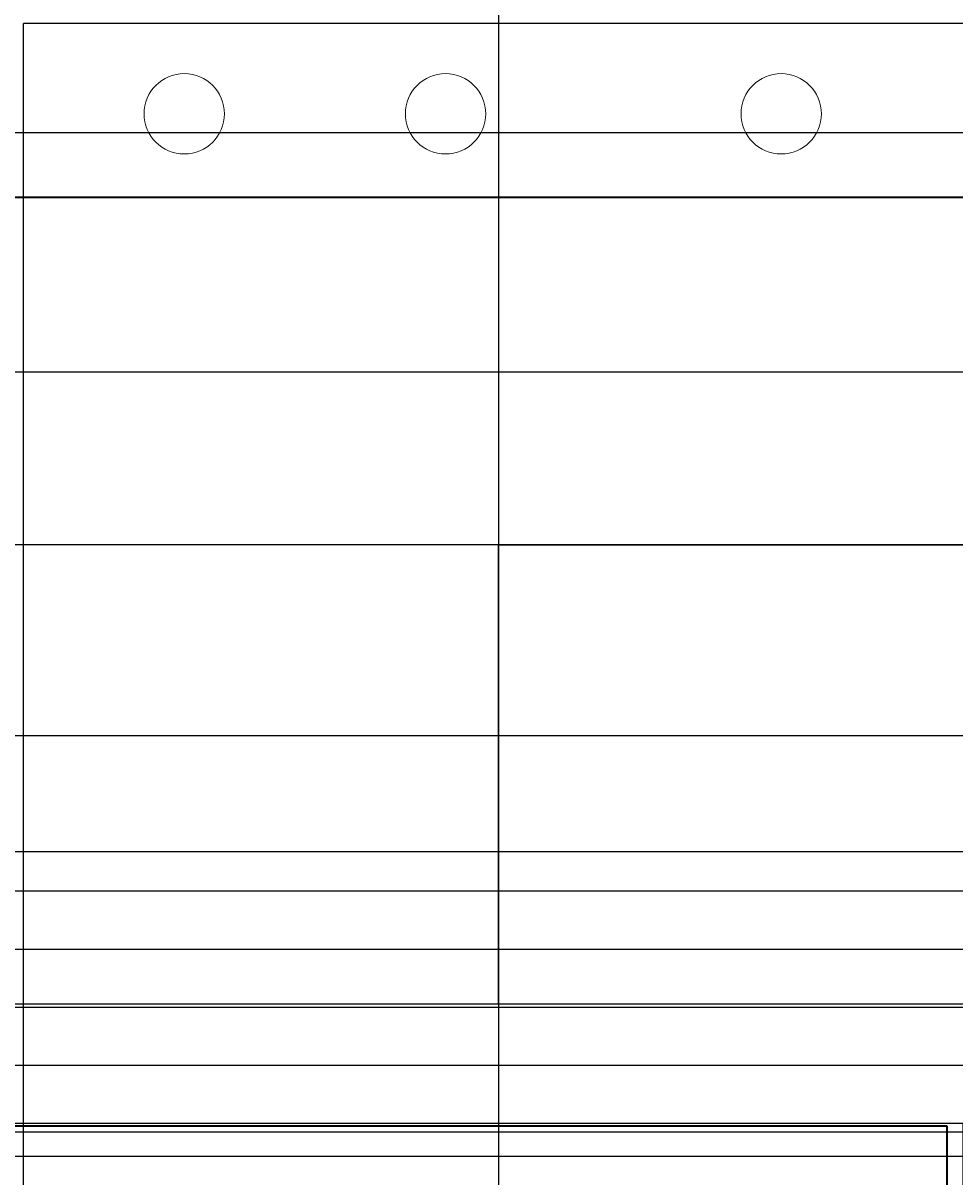
# Model space of a CAD drawing. Units: inches. Extents: x -13 to 809, y 112 to 656.
# Tile 10 of 55: x 161 to 257, y 205 to 325. Entities that reach past the tile are written whole.
import ezdxf

# ---------------------------------------------------------------- set-up
doc = ezdxf.new("R2010")
doc.units = ezdxf.units.IN
doc.header["$MEASUREMENT"] = 0
for name, color, linetype, lineweight in [('A-ANNO-DIMS', 2, 'Continuous', 18), ('A-ELEV', 7, 'Continuous', 35), ('A-ELEV-OTLN', 7, 'Continuous', 18), ('A-GLAZ', 4, 'Continuous', 25)]:
    doc.layers.add(name, color=color, linetype=linetype, lineweight=lineweight)
doc.styles.get("Standard").update_dxf_attribs({"font": 'arial.ttf'})
doc.dimstyles.get("Standard").update_dxf_attribs({"dimtxt": 0.625, "dimasz": 0.18, "dimexe": 0.18, "dimexo": 0.0625, "dimgap": 0.09, "dimtad": 0, "dimtih": 1, "dimtoh": 1, "dimdec": 4, "dimzin": 0, "dimdsep": 46, "dimlunit": 4, "dimtxsty": 'Standard', "dimcen": 0.09, "dimadec": 0, "dimazin": 0, "dimtfac": 1, "dimtdec": 4, "dimtofl": 0, "dimtmove": 0, "dimatfit": 3, "dimfxl": 1, "dimtolj": 1, "dimtzin": 0, "dimarcsym": 0})

# ---------------------------------------------------------------- blocks, each defined once
blk = doc.blocks.new('*D13')
at = {"layer": 'A-ANNO-DIMS', "color": 0, "lineweight": -2, "transparency": 16777216}
for p, q in [((124.92, 210.46), (124.92, 112.34)), ((160.92, 210.46), (160.92, 112.34)), ((125.1, 112.52), (142.38, 112.52)), ((160.74, 112.52), (143.46, 112.52))]:
    blk.add_line(p, q, dxfattribs=at)
at = {"layer": 'A-ANNO-DIMS', "color": 0, "transparency": 16777216}
for points in [[(125.1, 112.55), (125.1, 112.49), (124.92, 112.52)], [(160.74, 112.55), (160.74, 112.49), (160.92, 112.52)]]:
    blk.add_solid(points, dxfattribs=at)
at = {"layer": 'Defpoints', "color": 0, "transparency": 16777216}
for p in [(124.92, 210.52), (160.92, 210.52), (160.92, 112.52)]:
    blk.add_point(p, dxfattribs=at)
at = {"layer": 'A-ANNO-DIMS', "color": 0, "transparency": 16777216, "insert": (142.92, 112.52), "char_height": 0.625, "attachment_point": 5}
blk.add_mtext('\\A1;36', dxfattribs=at)
blk = doc.blocks.new('*D14')
at = {"layer": 'A-ANNO-DIMS', "color": 0, "lineweight": -2, "transparency": 16777216}
for p, q in [((210.08, 223.04), (210.08, 112.34)), ((160.92, 210.46), (160.92, 112.34)), ((161.1, 112.52), (184.34, 112.52)), ((209.9, 112.52), (186.66, 112.52))]:
    blk.add_line(p, q, dxfattribs=at)
at = {"layer": 'A-ANNO-DIMS', "color": 0, "transparency": 16777216}
for points in [[(161.1, 112.55), (161.1, 112.49), (160.92, 112.52)], [(209.9, 112.55), (209.9, 112.49), (210.08, 112.52)]]:
    blk.add_solid(points, dxfattribs=at)
at = {"layer": 'Defpoints', "color": 0, "transparency": 16777216}
for p in [(210.08, 223.1), (160.92, 210.52), (210.08, 112.52)]:
    blk.add_point(p, dxfattribs=at)
at = {"layer": 'A-ANNO-DIMS', "color": 0, "transparency": 16777216, "insert": (185.5, 112.52), "char_height": 0.625, "attachment_point": 5}
blk.add_mtext('\\A1;49.16', dxfattribs=at)
blk = doc.blocks.new('*D15')
at = {"layer": 'A-ANNO-DIMS', "color": 0, "lineweight": -2, "transparency": 16777216}
for p, q in [((210.08, 223.04), (210.08, 112.34)), ((258.1, 210.72), (258.1, 112.34)), ((210.26, 112.52), (232.94, 112.52)), ((257.92, 112.52), (235.24, 112.52))]:
    blk.add_line(p, q, dxfattribs=at)
at = {"layer": 'A-ANNO-DIMS', "color": 0, "transparency": 16777216}
for points in [[(210.26, 112.55), (210.26, 112.49), (210.08, 112.52)], [(257.92, 112.55), (257.92, 112.49), (258.1, 112.52)]]:
    blk.add_solid(points, dxfattribs=at)
at = {"layer": 'Defpoints', "color": 0, "transparency": 16777216}
for p in [(210.08, 223.1), (258.1, 210.78), (258.1, 112.52)]:
    blk.add_point(p, dxfattribs=at)
at = {"layer": 'A-ANNO-DIMS', "color": 0, "transparency": 16777216, "insert": (234.09, 112.52), "char_height": 0.625, "attachment_point": 5}
blk.add_mtext('\\A1;48.02', dxfattribs=at)
blk = doc.blocks.new('*D39')
at = {"layer": 'A-ANNO-DIMS', "color": 0, "lineweight": -2, "transparency": 16777216}
for p, q in [((341.34, 524.28), (-12.1, 524.28)), ((-11.92, 524.1), (-11.92, 406.78)), ((-11.92, 288.63), (-11.92, 405.96)), ((341.34, 288.45), (-12.1, 288.45))]:
    blk.add_line(p, q, dxfattribs=at)
at = {"layer": 'A-ANNO-DIMS', "color": 0, "transparency": 16777216}
for points in [[(-11.95, 524.1), (-11.89, 524.1), (-11.92, 524.28)], [(-11.95, 288.63), (-11.89, 288.63), (-11.92, 288.45)]]:
    blk.add_solid(points, dxfattribs=at)
at = {"layer": 'Defpoints', "color": 0, "transparency": 16777216}
for p in [(-11.92, 524.28), (341.41, 524.28), (341.41, 288.45)]:
    blk.add_point(p, dxfattribs=at)
at = {"layer": 'A-ANNO-DIMS', "color": 0, "transparency": 16777216, "insert": (-11.92, 406.37), "char_height": 0.625, "attachment_point": 5}
blk.add_mtext('\\A1;235.83', dxfattribs=at)
blk = doc.blocks.new('*D40')
at = {"layer": 'A-ANNO-DIMS', "color": 0, "lineweight": -2, "transparency": 16777216}
for p, q in [((471.04, 313.17), (-12.1, 313.17)), ((-11.92, 312.99), (-11.92, 301.22)), ((-11.92, 288.63), (-11.92, 300.4)), ((341.34, 288.45), (-12.1, 288.45))]:
    blk.add_line(p, q, dxfattribs=at)
at = {"layer": 'A-ANNO-DIMS', "color": 0, "transparency": 16777216}
for points in [[(-11.95, 312.99), (-11.89, 312.99), (-11.92, 313.17)], [(-11.95, 288.63), (-11.89, 288.63), (-11.92, 288.45)]]:
    blk.add_solid(points, dxfattribs=at)
at = {"layer": 'Defpoints', "color": 0, "transparency": 16777216}
for p in [(471.1, 313.17), (-11.92, 288.45), (341.41, 288.45)]:
    blk.add_point(p, dxfattribs=at)
at = {"layer": 'A-ANNO-DIMS', "color": 0, "transparency": 16777216, "insert": (-11.92, 300.81), "char_height": 0.625, "attachment_point": 5}
blk.add_mtext('\\A1;24.716', dxfattribs=at)
blk = doc.blocks.new('*D41')
at = {"layer": 'A-ANNO-DIMS', "color": 0, "lineweight": -2, "transparency": 16777216}
for p, q in [((471.04, 357.98), (-12.1, 357.98)), ((-11.92, 357.8), (-11.92, 335.98)), ((-11.92, 313.35), (-11.92, 335.16)), ((471.04, 313.17), (-12.1, 313.17))]:
    blk.add_line(p, q, dxfattribs=at)
at = {"layer": 'A-ANNO-DIMS', "color": 0, "transparency": 16777216}
for points in [[(-11.95, 357.8), (-11.89, 357.8), (-11.92, 357.98)], [(-11.95, 313.35), (-11.89, 313.35), (-11.92, 313.17)]]:
    blk.add_solid(points, dxfattribs=at)
at = {"layer": 'Defpoints', "color": 0, "transparency": 16777216}
for p in [(-11.92, 357.98), (471.1, 357.98), (471.1, 313.17)]:
    blk.add_point(p, dxfattribs=at)
at = {"layer": 'A-ANNO-DIMS', "color": 0, "transparency": 16777216, "insert": (-11.92, 335.57), "char_height": 0.625, "attachment_point": 5}
blk.add_mtext('\\A1;44.81', dxfattribs=at)
blk = doc.blocks.new('*D45')
at = {"layer": 'A-ANNO-DIMS', "color": 0, "lineweight": -2, "transparency": 16777216}
for p, q in [((275.65, 270.6), (-12.1, 270.6)), ((-11.92, 270.42), (-11.92, 247.26)), ((-11.92, 223.28), (-11.92, 246.44)), ((275.65, 223.1), (-12.1, 223.1))]:
    blk.add_line(p, q, dxfattribs=at)
at = {"layer": 'A-ANNO-DIMS', "color": 0, "transparency": 16777216}
for points in [[(-11.95, 270.42), (-11.89, 270.42), (-11.92, 270.6)], [(-11.95, 223.28), (-11.89, 223.28), (-11.92, 223.1)]]:
    blk.add_solid(points, dxfattribs=at)
at = {"layer": 'Defpoints', "color": 0, "transparency": 16777216}
for p in [(-11.92, 270.6), (275.71, 270.6), (275.71, 223.1)]:
    blk.add_point(p, dxfattribs=at)
at = {"layer": 'A-ANNO-DIMS', "color": 0, "transparency": 16777216, "insert": (-11.92, 246.85), "char_height": 0.625, "attachment_point": 5}
blk.add_mtext('\\A1;47.5', dxfattribs=at)
blk = doc.blocks.new('*D46')
at = {"layer": 'A-ANNO-DIMS', "color": 0, "lineweight": -2, "transparency": 16777216}
for p, q in [((160.98, 408.79), (807.77, 408.79)), ((807.59, 408.61), (807.59, 367.07)), ((807.59, 324.7), (807.59, 366.25)), ((160.98, 324.52), (807.77, 324.52))]:
    blk.add_line(p, q, dxfattribs=at)
at = {"layer": 'A-ANNO-DIMS', "color": 0, "transparency": 16777216}
for points in [[(807.56, 408.61), (807.62, 408.61), (807.59, 408.79)], [(807.56, 324.7), (807.62, 324.7), (807.59, 324.52)]]:
    blk.add_solid(points, dxfattribs=at)
at = {"layer": 'Defpoints', "color": 0, "transparency": 16777216}
for p in [(160.92, 408.79), (807.59, 408.79), (160.92, 324.52)]:
    blk.add_point(p, dxfattribs=at)
at = {"layer": 'A-ANNO-DIMS', "color": 0, "transparency": 16777216, "insert": (807.59, 366.66), "char_height": 0.625, "attachment_point": 5}
blk.add_mtext('\\A1;84.27', dxfattribs=at)
blk = doc.blocks.new('*D49')
at = {"layer": 'A-ANNO-DIMS', "color": 0, "lineweight": -2, "transparency": 16777216}
for p, q in [((590.95, 250.84), (-12.1, 250.84)), ((-11.92, 250.66), (-11.92, 245.25)), ((-11.92, 239.02), (-11.92, 244.44)), ((590.95, 238.84), (-12.1, 238.84))]:
    blk.add_line(p, q, dxfattribs=at)
at = {"layer": 'A-ANNO-DIMS', "color": 0, "transparency": 16777216}
for points in [[(-11.95, 250.66), (-11.89, 250.66), (-11.92, 250.84)], [(-11.95, 239.02), (-11.89, 239.02), (-11.92, 238.84)]]:
    blk.add_solid(points, dxfattribs=at)
at = {"layer": 'Defpoints', "color": 0, "transparency": 16777216}
for p in [(-11.92, 250.84), (591.01, 250.84), (591.01, 238.84)]:
    blk.add_point(p, dxfattribs=at)
at = {"layer": 'A-ANNO-DIMS', "color": 0, "transparency": 16777216, "insert": (-11.92, 244.84), "char_height": 0.625, "attachment_point": 5}
blk.add_mtext('\\A1;12', dxfattribs=at)
blk = doc.blocks.new('*D50')
at = {"layer": 'A-ANNO-DIMS', "color": 0, "lineweight": -2, "transparency": 16777216}
for p, q in [((590.95, 238.84), (-12.1, 238.84)), ((-11.92, 238.66), (-11.92, 224.77)), ((-11.92, 210.06), (-11.92, 223.95)), ((607.51, 209.88), (-12.1, 209.88))]:
    blk.add_line(p, q, dxfattribs=at)
at = {"layer": 'A-ANNO-DIMS', "color": 0, "transparency": 16777216}
for points in [[(-11.95, 238.66), (-11.89, 238.66), (-11.92, 238.84)], [(-11.95, 210.06), (-11.89, 210.06), (-11.92, 209.88)]]:
    blk.add_solid(points, dxfattribs=at)
at = {"layer": 'Defpoints', "color": 0, "transparency": 16777216}
for p in [(591.01, 238.84), (-11.92, 209.88), (607.57, 209.88)]:
    blk.add_point(p, dxfattribs=at)
at = {"layer": 'A-ANNO-DIMS', "color": 0, "transparency": 16777216, "insert": (-11.92, 224.36), "char_height": 0.625, "attachment_point": 5}
blk.add_mtext('\\A1;28.97', dxfattribs=at)
blk = doc.blocks.new('*D80')
at = {"layer": 'A-ANNO-DIMS', "color": 0, "lineweight": -2, "transparency": 16777216}
for p, q in [((368.83, 216.77), (-12.1, 216.77)), ((-11.92, 216.59), (-11.92, 214.18)), ((-11.92, 210.95), (-11.92, 213.36)), ((368.83, 210.77), (-12.1, 210.77))]:
    blk.add_line(p, q, dxfattribs=at)
at = {"layer": 'A-ANNO-DIMS', "color": 0, "transparency": 16777216}
for points in [[(-11.95, 216.59), (-11.89, 216.59), (-11.92, 216.77)], [(-11.95, 210.95), (-11.89, 210.95), (-11.92, 210.77)]]:
    blk.add_solid(points, dxfattribs=at)
at = {"layer": 'Defpoints', "color": 0, "transparency": 16777216}
for p in [(-11.92, 216.77), (368.9, 216.77), (368.9, 210.77)]:
    blk.add_point(p, dxfattribs=at)
at = {"layer": 'A-ANNO-DIMS', "color": 0, "transparency": 16777216, "insert": (-11.92, 213.77), "char_height": 0.625, "attachment_point": 5}
blk.add_mtext('\\A1;6', dxfattribs=at)
blk = doc.blocks.new('*D81')
at = {"layer": 'A-ANNO-DIMS', "color": 0, "lineweight": -2, "transparency": 16777216}
for p, q in [((378.83, 222.77), (-12.1, 222.77)), ((-11.92, 222.59), (-11.92, 220.18)), ((-11.92, 216.95), (-11.92, 219.36)), ((378.83, 216.77), (-12.1, 216.77))]:
    blk.add_line(p, q, dxfattribs=at)
at = {"layer": 'A-ANNO-DIMS', "color": 0, "transparency": 16777216}
for points in [[(-11.95, 222.59), (-11.89, 222.59), (-11.92, 222.77)], [(-11.95, 216.95), (-11.89, 216.95), (-11.92, 216.77)]]:
    blk.add_solid(points, dxfattribs=at)
at = {"layer": 'Defpoints', "color": 0, "transparency": 16777216}
for p in [(-11.92, 222.77), (378.9, 222.77), (378.9, 216.77)]:
    blk.add_point(p, dxfattribs=at)
at = {"layer": 'A-ANNO-DIMS', "color": 0, "transparency": 16777216, "insert": (-11.92, 219.77), "char_height": 0.625, "attachment_point": 5}
blk.add_mtext('\\A1;6', dxfattribs=at)
blk = doc.blocks.new('*D82')
at = {"layer": 'A-ANNO-DIMS', "color": 0, "lineweight": -2, "transparency": 16777216}
for p, q in [((388.83, 228.77), (-12.1, 228.77)), ((-11.92, 228.59), (-11.92, 226.18)), ((-11.92, 222.95), (-11.92, 225.36)), ((388.83, 222.77), (-12.1, 222.77))]:
    blk.add_line(p, q, dxfattribs=at)
at = {"layer": 'A-ANNO-DIMS', "color": 0, "transparency": 16777216}
for points in [[(-11.95, 228.59), (-11.89, 228.59), (-11.92, 228.77)], [(-11.95, 222.95), (-11.89, 222.95), (-11.92, 222.77)]]:
    blk.add_solid(points, dxfattribs=at)
at = {"layer": 'Defpoints', "color": 0, "transparency": 16777216}
for p in [(-11.92, 228.77), (388.9, 228.77), (388.9, 222.77)]:
    blk.add_point(p, dxfattribs=at)
at = {"layer": 'A-ANNO-DIMS', "color": 0, "transparency": 16777216, "insert": (-11.92, 225.77), "char_height": 0.625, "attachment_point": 5}
blk.add_mtext('\\A1;6', dxfattribs=at)
blk = doc.blocks.new('*D83')
at = {"layer": 'A-ANNO-DIMS', "color": 0, "lineweight": -2, "transparency": 16777216}
for p, q in [((398.83, 234.77), (-12.1, 234.77)), ((-11.92, 234.59), (-11.92, 232.18)), ((-11.92, 228.95), (-11.92, 231.36)), ((398.83, 228.77), (-12.1, 228.77))]:
    blk.add_line(p, q, dxfattribs=at)
at = {"layer": 'A-ANNO-DIMS', "color": 0, "transparency": 16777216}
for points in [[(-11.95, 234.59), (-11.89, 234.59), (-11.92, 234.77)], [(-11.95, 228.95), (-11.89, 228.95), (-11.92, 228.77)]]:
    blk.add_solid(points, dxfattribs=at)
at = {"layer": 'Defpoints', "color": 0, "transparency": 16777216}
for p in [(-11.92, 234.77), (398.9, 234.77), (398.9, 228.77)]:
    blk.add_point(p, dxfattribs=at)
at = {"layer": 'A-ANNO-DIMS', "color": 0, "transparency": 16777216, "insert": (-11.92, 231.77), "char_height": 0.625, "attachment_point": 5}
blk.add_mtext('\\A1;6', dxfattribs=at)
blk = doc.blocks.new('*D84')
at = {"layer": 'A-ANNO-DIMS', "color": 0, "lineweight": -2, "transparency": 16777216}
for p, q in [((408.83, 238.84), (-12.1, 238.84)), ((-11.92, 238.66), (-11.92, 237.22)), ((-11.92, 234.95), (-11.92, 236.4)), ((408.83, 234.77), (-12.1, 234.77))]:
    blk.add_line(p, q, dxfattribs=at)
at = {"layer": 'A-ANNO-DIMS', "color": 0, "transparency": 16777216}
for points in [[(-11.95, 238.66), (-11.89, 238.66), (-11.92, 238.84)], [(-11.95, 234.95), (-11.89, 234.95), (-11.92, 234.77)]]:
    blk.add_solid(points, dxfattribs=at)
at = {"layer": 'Defpoints', "color": 0, "transparency": 16777216}
for p in [(-11.92, 238.84), (408.9, 238.84), (408.9, 234.77)]:
    blk.add_point(p, dxfattribs=at)
at = {"layer": 'A-ANNO-DIMS', "color": 0, "transparency": 16777216, "insert": (-11.92, 236.81), "char_height": 0.625, "attachment_point": 5}
blk.add_mtext('\\A1;4.069', dxfattribs=at)
blk = doc.blocks.new('*D94')
at = {"layer": 'A-ANNO-DIMS', "color": 0, "lineweight": -2, "transparency": 16777216}
for p, q in [((210.02, 223.1), (-12.1, 223.1)), ((-11.92, 222.92), (-11.92, 217.22)), ((-11.92, 210.7), (-11.92, 216.4)), ((160.86, 210.52), (-12.1, 210.52))]:
    blk.add_line(p, q, dxfattribs=at)
at = {"layer": 'A-ANNO-DIMS', "color": 0, "transparency": 16777216}
for points in [[(-11.95, 222.92), (-11.89, 222.92), (-11.92, 223.1)], [(-11.95, 210.7), (-11.89, 210.7), (-11.92, 210.52)]]:
    blk.add_solid(points, dxfattribs=at)
at = {"layer": 'Defpoints', "color": 0, "transparency": 16777216}
for p in [(-11.92, 223.1), (210.08, 223.1), (160.92, 210.52)]:
    blk.add_point(p, dxfattribs=at)
at = {"layer": 'A-ANNO-DIMS', "color": 0, "transparency": 16777216, "insert": (-11.92, 216.81), "char_height": 0.625, "attachment_point": 5}
blk.add_mtext('\\A1;12.58', dxfattribs=at)
blk = doc.blocks.new('*D110')
at = {"layer": 'A-ANNO-DIMS', "color": 0, "lineweight": -2, "transparency": 16777216}
for p, q in [((124.92, 324.46), (124.92, 112.34)), ((160.92, 324.46), (160.92, 112.34)), ((125.1, 112.52), (141.78, 112.52)), ((160.74, 112.52), (144.06, 112.52))]:
    blk.add_line(p, q, dxfattribs=at)
at = {"layer": 'A-ANNO-DIMS', "color": 0, "transparency": 16777216}
for points in [[(125.1, 112.55), (125.1, 112.49), (124.92, 112.52)], [(160.74, 112.55), (160.74, 112.49), (160.92, 112.52)]]:
    blk.add_solid(points, dxfattribs=at)
at = {"layer": 'Defpoints', "color": 0, "transparency": 16777216}
for p in [(124.92, 324.52), (160.92, 324.52), (160.92, 112.52)]:
    blk.add_point(p, dxfattribs=at)
at = {"layer": 'A-ANNO-DIMS', "color": 0, "transparency": 16777216, "insert": (142.92, 112.52), "char_height": 0.625, "attachment_point": 5}
blk.add_mtext('\\A1;36.00', dxfattribs=at)
blk = doc.blocks.new('*D111')
at = {"layer": 'A-ANNO-DIMS', "color": 0, "lineweight": -2, "transparency": 16777216}
for p, q in [((210.08, 361.23), (210.08, 112.34)), ((160.92, 324.46), (160.92, 112.34)), ((161.1, 112.52), (184.34, 112.52)), ((209.9, 112.52), (186.66, 112.52))]:
    blk.add_line(p, q, dxfattribs=at)
at = {"layer": 'A-ANNO-DIMS', "color": 0, "transparency": 16777216}
for points in [[(161.1, 112.55), (161.1, 112.49), (160.92, 112.52)], [(209.9, 112.55), (209.9, 112.49), (210.08, 112.52)]]:
    blk.add_solid(points, dxfattribs=at)
at = {"layer": 'Defpoints', "color": 0, "transparency": 16777216}
for p in [(210.08, 361.29), (160.92, 324.52), (210.08, 112.52)]:
    blk.add_point(p, dxfattribs=at)
at = {"layer": 'A-ANNO-DIMS', "color": 0, "transparency": 16777216, "insert": (185.5, 112.52), "char_height": 0.625, "attachment_point": 5}
blk.add_mtext('\\A1;49.16', dxfattribs=at)
blk = doc.blocks.new('*D112')
at = {"layer": 'A-ANNO-DIMS', "color": 0, "lineweight": -2, "transparency": 16777216}
for p, q in [((210.08, 361.23), (210.08, 112.34)), ((275.71, 361.23), (275.71, 112.34)), ((210.26, 112.52), (241.75, 112.52)), ((275.53, 112.52), (244.04, 112.52))]:
    blk.add_line(p, q, dxfattribs=at)
at = {"layer": 'A-ANNO-DIMS', "color": 0, "transparency": 16777216}
for points in [[(210.26, 112.55), (210.26, 112.49), (210.08, 112.52)], [(275.53, 112.55), (275.53, 112.49), (275.71, 112.52)]]:
    blk.add_solid(points, dxfattribs=at)
at = {"layer": 'Defpoints', "color": 0, "transparency": 16777216}
for p in [(210.08, 361.29), (275.71, 361.29), (275.71, 112.52)]:
    blk.add_point(p, dxfattribs=at)
at = {"layer": 'A-ANNO-DIMS', "color": 0, "transparency": 16777216, "insert": (242.9, 112.52), "char_height": 0.625, "attachment_point": 5}
blk.add_mtext('\\A1;65.64', dxfattribs=at)
blk = doc.blocks.new('*D115')
at = {"layer": 'A-ANNO-DIMS', "color": 0, "lineweight": -2, "transparency": 16777216}
for p, q in [((311.4, 210.78), (-12.1, 210.78)), ((-11.92, 210.6), (-11.92, 181.06)), ((-11.92, 150.7), (-11.92, 180.24)), ((311.64, 150.52), (-12.1, 150.52))]:
    blk.add_line(p, q, dxfattribs=at)
at = {"layer": 'A-ANNO-DIMS', "color": 0, "transparency": 16777216}
for points in [[(-11.95, 210.6), (-11.89, 210.6), (-11.92, 210.78)], [(-11.95, 150.7), (-11.89, 150.7), (-11.92, 150.52)]]:
    blk.add_solid(points, dxfattribs=at)
at = {"layer": 'Defpoints', "color": 0, "transparency": 16777216}
for p in [(-11.92, 210.78), (311.46, 210.78), (311.7, 150.52)]:
    blk.add_point(p, dxfattribs=at)
at = {"layer": 'A-ANNO-DIMS', "color": 0, "transparency": 16777216, "insert": (-11.92, 180.65), "char_height": 0.625, "attachment_point": 5}
blk.add_mtext('\\A1;60.27', dxfattribs=at)
blk = doc.blocks.new('*D118')
at = {"layer": 'A-ANNO-DIMS', "color": 0, "lineweight": -2, "transparency": 16777216}
for p, q in [((311.4, 210.78), (-12.1, 210.78)), ((-11.92, 210.6), (-11.92, 209.49)), ((-11.92, 207.55), (-11.92, 208.67)), ((308.59, 207.37), (-12.1, 207.37))]:
    blk.add_line(p, q, dxfattribs=at)
at = {"layer": 'A-ANNO-DIMS', "color": 0, "transparency": 16777216}
for points in [[(-11.95, 210.6), (-11.89, 210.6), (-11.92, 210.78)], [(-11.95, 207.55), (-11.89, 207.55), (-11.92, 207.37)]]:
    blk.add_solid(points, dxfattribs=at)
at = {"layer": 'Defpoints', "color": 0, "transparency": 16777216}
for p in [(-11.92, 210.78), (311.46, 210.78), (308.65, 207.37)]:
    blk.add_point(p, dxfattribs=at)
at = {"layer": 'A-ANNO-DIMS', "color": 0, "transparency": 16777216, "insert": (-11.92, 209.08), "char_height": 0.625, "attachment_point": 5}
blk.add_mtext('\\A1;3.41', dxfattribs=at)

msp = doc.modelspace()

# ---------------------------------------------------------------- linework, layer by layer
at = {"layer": 'A-ELEV'}
for p, q in [((109.5888, 306.5199), (337.5074, 306.5199)), ((26.0809, 210.5199), (256.4464, 210.5199)), ((256.4464, 210.5199), (256.4464, 150.5199))]:
    msp.add_line(p, q, dxfattribs=at)
at = {"layer": 'A-ELEV-OTLN'}
for centre in [(177.5857, 315.1435), (204.6029, 315.1435), (239.3079, 315.1435)]:
    msp.add_circle(centre, 4.1542, dxfattribs=at)
at = {"layer": 'A-GLAZ'}
msp.add_lwpolyline([(210.0791, 270.6024), (275.7145, 270.6024), (275.7145, 223.1), (210.0791, 223.1)], close=True, dxfattribs=at)

# ---------------------------------------------------------------- dimensions: what is measured, and where the dimension line sits
at = {"layer": 'A-ANNO-DIMS'}
for base, p1, p2, override, picture, middle in [((-11.9191, 524.281), (341.4072, 288.4508), (341.4072, 524.281), {"dimdec": 2, "dimlfac": 1, "dimrnd": 0, "dimzin": 0, "dimdsep": 46, "dimlunit": 2}, '*D39', (-11.9191, 406.3659)), ((807.5888, 408.7939), (160.9184, 324.5199), (160.9184, 408.7939), {"dimdec": 2, "dimlfac": 1, "dimrnd": 0, "dimzin": 0, "dimdsep": 46, "dimlunit": 2}, '*D46', (807.5888, 366.6569)), ((-11.9191, 357.9804), (471.0998, 313.1667), (471.0998, 357.9804), {"dimdec": 2, "dimlfac": 1, "dimrnd": 0, "dimzin": 0, "dimdsep": 46, "dimlunit": 2}, '*D41', (-11.9191, 335.5735)), ((-11.9191, 288.4508), (471.0998, 313.1667), (341.4072, 288.4508), {"dimdec": 3, "dimlfac": 1, "dimrnd": 0, "dimzin": 0, "dimdsep": 46, "dimlunit": 2}, '*D40', (-11.9191, 300.8087)), ((-11.9191, 270.6024), (275.7145, 223.1), (275.7145, 270.6024), {"dimdec": 1, "dimlfac": 1, "dimrnd": 0, "dimzin": 0, "dimdsep": 46, "dimlunit": 2}, '*D45', (-11.9191, 246.8512)), ((-11.9191, 250.8429), (591.008, 238.8429), (591.008, 250.8429), {"dimdec": 0, "dimlfac": 1, "dimrnd": 0, "dimzin": 0, "dimdsep": 46, "dimlunit": 2}, '*D49', (-11.9191, 244.8429)), ((-11.9191, 209.8753), (591.008, 238.8429), (607.5741, 209.8753), {"dimdec": 2, "dimlfac": 1, "dimrnd": 0, "dimzin": 0, "dimdsep": 46, "dimlunit": 2}, '*D50', (-11.9191, 224.3591)), ((-11.9191, 238.8429), (408.8966, 234.7738), (408.8966, 238.8429), {"dimdec": 3, "dimlfac": 1, "dimrnd": 0, "dimzin": 0, "dimdsep": 46, "dimlunit": 2}, '*D84', (-11.9191, 236.8083)), ((-11.9191, 234.7738), (398.8966, 228.7738), (398.8966, 234.7738), {"dimdec": 0, "dimlfac": 1, "dimrnd": 0, "dimzin": 0, "dimdsep": 46, "dimlunit": 2}, '*D83', (-11.9191, 231.7738)), ((-11.9191, 228.7738), (388.8966, 222.7738), (388.8966, 228.7738), {"dimdec": 0, "dimlfac": 1, "dimrnd": 0, "dimzin": 0, "dimdsep": 46, "dimlunit": 2}, '*D82', (-11.9191, 225.7738)), ((-11.9191, 223.1), (160.9184, 210.5199), (210.0791, 223.1), {"dimdec": 2, "dimlfac": 1, "dimrnd": 0, "dimzin": 0, "dimdsep": 46, "dimlunit": 2}, '*D94', (-11.9191, 216.81)), ((-11.9191, 222.7738), (378.8966, 216.7738), (378.8966, 222.7738), {"dimdec": 0, "dimlfac": 1, "dimrnd": 0, "dimzin": 0, "dimdsep": 46, "dimlunit": 2}, '*D81', (-11.9191, 219.7738)), ((-11.9191, 216.7738), (368.8966, 210.7738), (368.8966, 216.7738), {"dimdec": 0, "dimlfac": 1, "dimrnd": 0, "dimzin": 0, "dimdsep": 46, "dimlunit": 2}, '*D80', (-11.9191, 213.7738)), ((-11.91915, 210.78493), (311.6991, 150.51989), (311.46269, 210.78493), {"dimdec": 2, "dimlfac": 1, "dimrnd": 0, "dimzin": 0, "dimdsep": 46, "dimlunit": 2}, '*D115', (-11.91915, 180.65241)), ((-11.9191, 210.7849), (308.6488, 207.3724), (311.4627, 210.7849), {"dimdec": 2, "dimlfac": 1, "dimrnd": 0, "dimzin": 0, "dimdsep": 46, "dimlunit": 2}, '*D118', (-11.9191, 209.0787))]:
    dim = msp.add_linear_dim(base=base, p1=p1, p2=p2, angle=90, dimstyle='Standard', override=override, dxfattribs=at)
    dim.commit()
    dim.dimension.update_dxf_attribs({"geometry": picture, "text_midpoint": middle})
for base, p1, p2, override, picture, middle in [((210.0791, 112.5199), (160.9184, 324.5199), (210.0791, 361.2915), {"dimdec": 2, "dimlfac": 1, "dimrnd": 0, "dimzin": 0, "dimdsep": 46, "dimlunit": 2}, '*D111', (185.4988, 112.5199)), ((275.7145, 112.5199), (210.0791, 361.2915), (275.7145, 361.2915), {"dimdec": 2, "dimlfac": 1, "dimrnd": 0, "dimzin": 0, "dimdsep": 46, "dimlunit": 2}, '*D112', (242.8968, 112.5199)), ((160.9184, 112.5199), (124.9184, 324.5199), (160.9184, 324.5199), {"dimdec": 2, "dimlfac": 1, "dimrnd": 0, "dimzin": 0, "dimdsep": 46, "dimlunit": 2}, '*D110', (142.9184, 112.5199)), ((210.0791, 112.5199), (160.9184, 210.5199), (210.0791, 223.1), {"dimdec": 2, "dimlfac": 1, "dimrnd": 0, "dimzin": 0, "dimdsep": 46, "dimlunit": 2}, '*D14', (185.4988, 112.5199)), ((258.1022, 112.5199), (210.0791, 223.1), (258.1022, 210.7849), {"dimdec": 2, "dimlfac": 1, "dimrnd": 0, "dimzin": 0, "dimdsep": 46, "dimlunit": 2}, '*D15', (234.0906, 112.5199)), ((160.9184, 112.5199), (124.9184, 210.5199), (160.9184, 210.5199), {"dimdec": 0, "dimlfac": 1, "dimrnd": 0, "dimzin": 0, "dimdsep": 46, "dimlunit": 2}, '*D13', (142.9184, 112.5199))]:
    dim = msp.add_linear_dim(base=base, p1=p1, p2=p2, dimstyle='Standard', override=override, dxfattribs=at)
    dim.commit()
    dim.dimension.update_dxf_attribs({"geometry": picture, "text_midpoint": middle})

doc.saveas('drawing.dxf')
